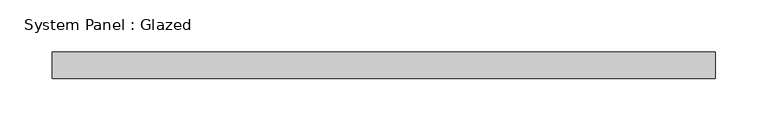
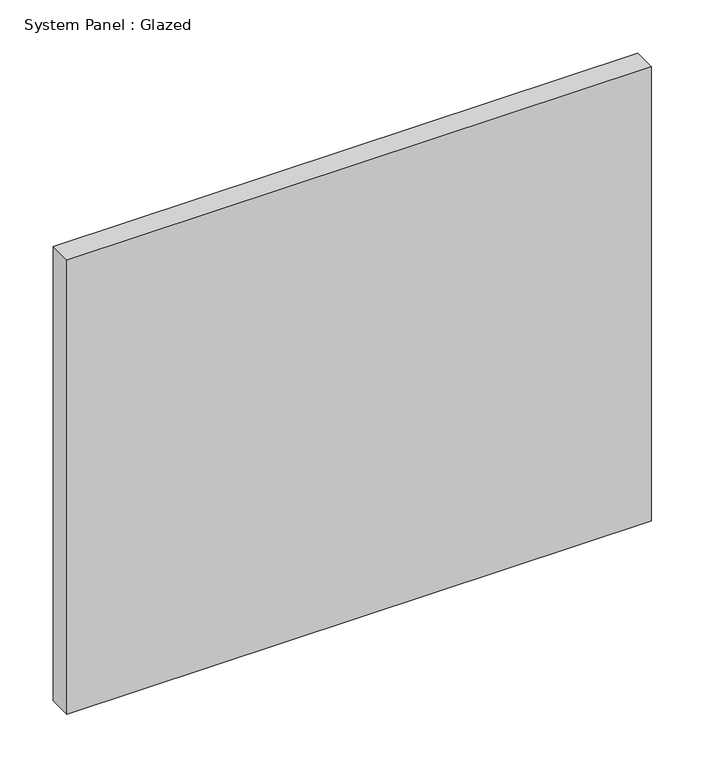
"""IFC4 building model written with IfcOpenShell, lengths in millimetres: plate geometry, System Panel : Glazed."""

from ifc_helpers import new_model, si_unit, origin, origin_with_axes, place, context, project, spatial, polyline, outline, extrude, source, transform, mapped, element, save


def system_panel_glazed_5707a053(model_context):
    return source(origin(), model_context, "Body", "SweptSolid", [
        extrude(outline(polyline([(317.5, 19.05), (-317.5, 19.05), (-317.5, 44.45), (317.5, 44.45), (317.5, 19.05)])), origin_with_axes(), (0.0, 0.0, 1.0), 521.9848788),
    ])


if __name__ == "__main__":
    model = new_model("IFC4")
    model_context = context("Model", 3, world=origin())
    ifc_project = project(units=[si_unit("LENGTHUNIT", "METRE", prefix="MILLI")], contexts=[model_context])
    site = spatial("IfcSite", under=ifc_project)
    building = spatial("IfcBuilding", under=site)
    placement = place(None, origin())
    system_panel_glazed_shape = system_panel_glazed_5707a053(model_context)
    element("IfcPlate", 1, ObjectType="System Panel : Glazed", at=placement, inside=building, context=model_context, shape_type="MappedRepresentation", body=[
        mapped(system_panel_glazed_shape, transform((0.0, 0.0, 0.0), x_axis=(1.0, 0.0, 0.0), y_axis=(0.0, 1.0, 0.0), z_axis=(0.0, 0.0, 1.0))),
    ])
    save(model, "model.ifc")

# Revit data of these elements
# Type "System Panel : Glazed"
#   Construction Type Id = "GSP4R"
#   Analytic Construction = "1/8 in Pilkington single glazing"
#   Visual Light Transmittance = 0.9
#   Solar Heat Gain Coefficient = 0.86
#   Heat Transfer Coefficient (U) = 1.18115 BTU/(h·ft²·°F)
#   Define Thermal Properties by = 1
# Element 1 (IfcPlate, "System Panel : Glazed")
#   Materials on its faces: "Glass"
# Materials
#   "Glass": class "Glass", colour RGB 0 128 192, transparency 0.75, Description = "Soda Lime Glass", Cost = 0
